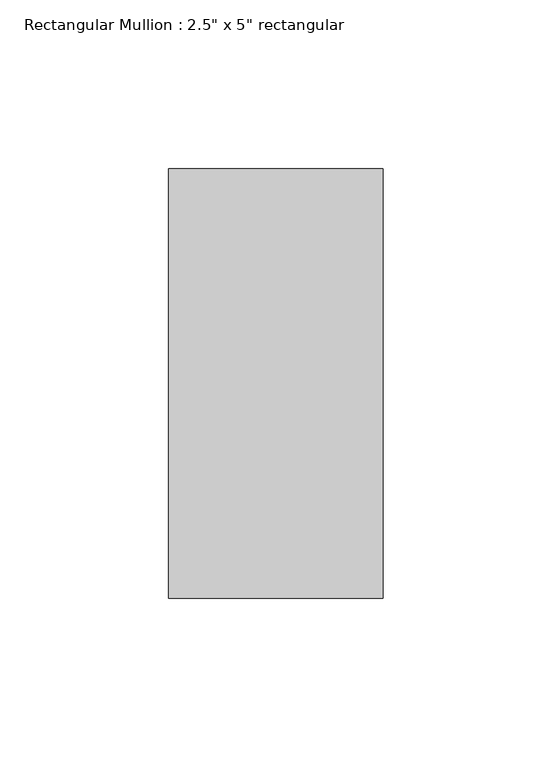
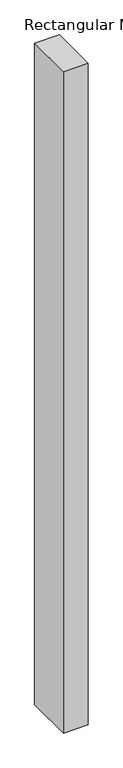
"""IFC4 building model written with IfcOpenShell, lengths in millimetres: member geometry."""

from ifc_helpers import new_model, si_unit, frame, origin, place, context, project, spatial, polyline, outline, extrude, source, transform, mapped, element, save


def member_3054d540(model_context):
    return source(origin(), model_context, "Body", "SweptSolid", [
        extrude(outline(polyline([(31.75, 63.5), (31.75, -63.5), (-31.75, -63.5), (-31.75, 63.5), (31.75, 63.5)])), frame((0.0, 0.0, -1792.8537153), z_axis=(0.0, 0.0, 1.0), x_axis=(1.0, 0.0, 0.0)), (0.0, 0.0, 1.0), 1792.8537153),
    ])


if __name__ == "__main__":
    model = new_model("IFC4")
    model_context = context("Model", 3, world=origin())
    ifc_project = project(units=[si_unit("LENGTHUNIT", "METRE", prefix="MILLI")], contexts=[model_context])
    site = spatial("IfcSite", under=ifc_project)
    building = spatial("IfcBuilding", under=site)
    placement = place(None, origin())
    member_shape = member_3054d540(model_context)
    element("IfcMember", 1, ObjectType="Rectangular Mullion : 2.5\" x 5\" rectangular", at=placement, inside=building, context=model_context, shape_type="MappedRepresentation", body=[
        mapped(member_shape, transform((0.0, 0.0, 0.0), x_axis=(1.0, 0.0, 0.0), y_axis=(0.0, 1.0, 0.0), z_axis=(0.0, 0.0, 1.0))),
    ])
    save(model, "model.ifc")

# Revit data of these elements
# Type "Rectangular Mullion : 2.5\" x 5\" rectangular"
#   built-in parameter 1007304 = 0.416667 (stored number, unit not read)
#   built-in parameter 1007301 = 0.104167 (stored number, unit not read)
#   built-in parameter 1007300 = 0.104167 (stored number, unit not read)
# Element 1 (IfcMember, "Rectangular Mullion : 2.5\" x 5\" rectangular")
#   Materials on its faces: "Aluminum"
# Materials
#   "Aluminum": class "Metal", colour RGB 247 247 247, transparency 0, Description = "Aluminum 6061", Cost = 0
